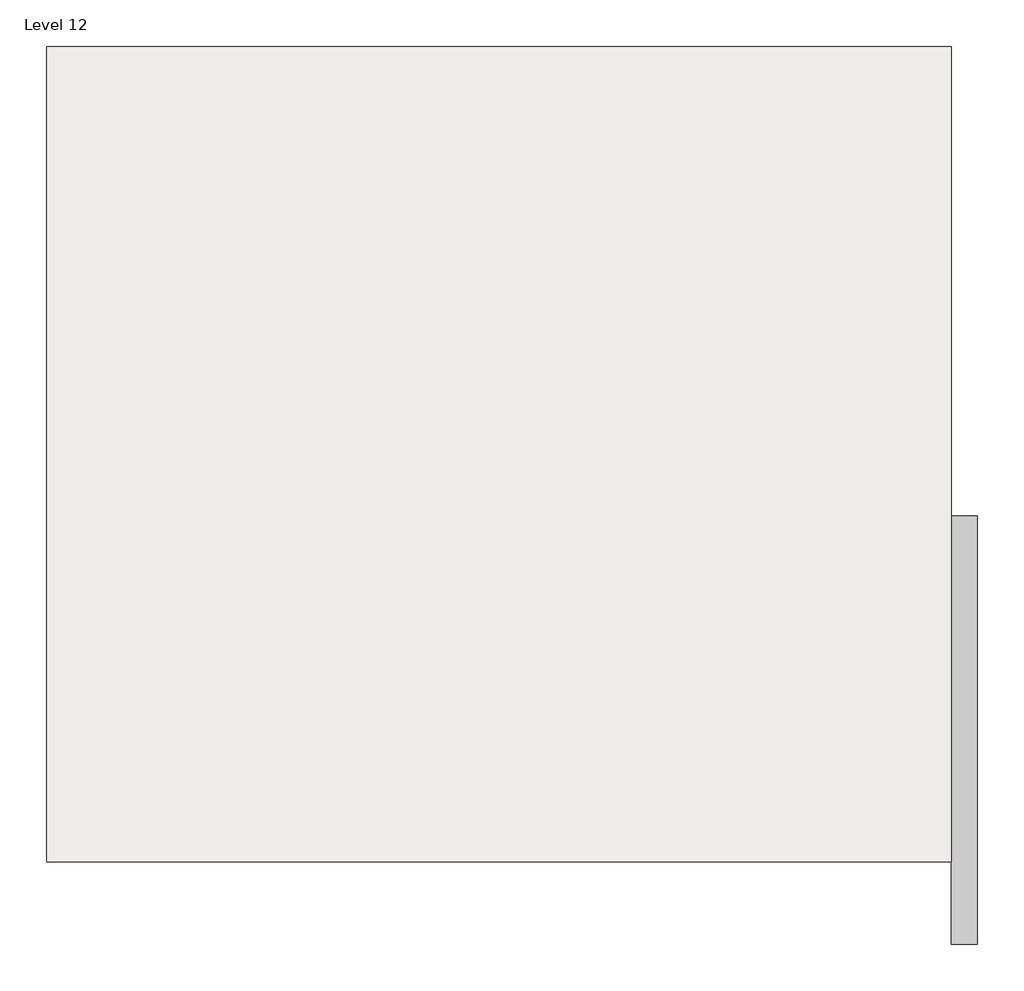
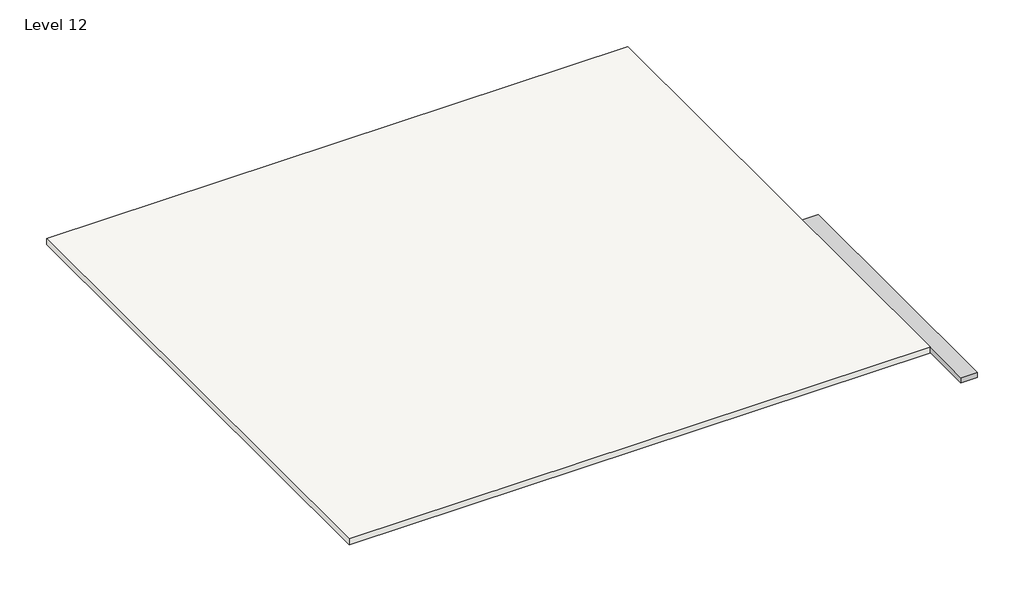
# One storey: 1 proxy, 1 slab.
"""IFC4 building model written with IfcOpenShell, lengths in millimetres."""

from ifc_helpers import new_model, si_unit, frame, origin, place, context, project, spatial, polyline, outline, extrude, transform, mapped, element, save
from components import generic_models_1_generic_models_1_103236ad

model = new_model("IFC4")

# Units and contexts
model_context = context("Model", 3, world=origin())
ifc_project = project(units=[si_unit("LENGTHUNIT", "METRE", prefix="MILLI")], contexts=[model_context])

# Site, building, storey
site = spatial("IfcSite", under=ifc_project)
building = spatial("IfcBuilding", under=site)
storey = spatial("IfcBuildingStorey", under=building, Name="Level 12", Elevation=18592.8)

# Proxy
placement = place(None, origin())
generic_models_1_generic_models_1_shape = generic_models_1_generic_models_1_103236ad(model_context)
element("IfcBuildingElementProxy", 1, Name="Generic Models 1 : Generic Models 1", ObjectType="Generic Models 1 : Generic Models 1", at=placement, inside=storey, context=model_context, shape_type="MappedRepresentation", body=[
    mapped(generic_models_1_generic_models_1_shape, transform((0.0, -228.6, 76.2), x_axis=(1.0, 0.0, 0.0), y_axis=(0.0, 1.0, 0.0), z_axis=(0.0, 0.0, 1.0))),
])

# Slab
element("IfcSlab", 2, ObjectType="Generic - 12\"", at=placement, inside=storey, context=model_context, shape_type="SweptSolid", body=[
    extrude(outline(polyline([(14106.5361222, 14825.1934186), (14106.5361222, -10371.6065814), (-13833.4638778, -10371.6065814), (-13833.4638778, 14825.1934186), (14106.5361222, 14825.1934186)])), frame((0.0, 0.0, 18613.9849443), z_axis=(0.0, 0.0, 1.0), x_axis=(1.0, 0.0, 0.0)), (0.0, 0.0, 1.0), 304.8),
])

save(model, "model.ifc")

# Revit data of these elements
# Type "Generic - 12\""
#   Assembly Code = "B1010"
#   Function = 0
#   Layers, outside or top first: 1' - 0" no material (function 1)
# Element 1 (IfcBuildingElementProxy, "Generic Models 1 : Generic Models 1")
#   Phase Created = New Construction
# Element 2 (IfcSlab, "Generic - 12\"")
#   Height Offset From Level = 1' - 0.83405"
#   Phase Created = New Construction
#   Materials on its faces: "Default Floor"
# Materials
#   "Default Floor": colour RGB 128 128 128, transparency 0
